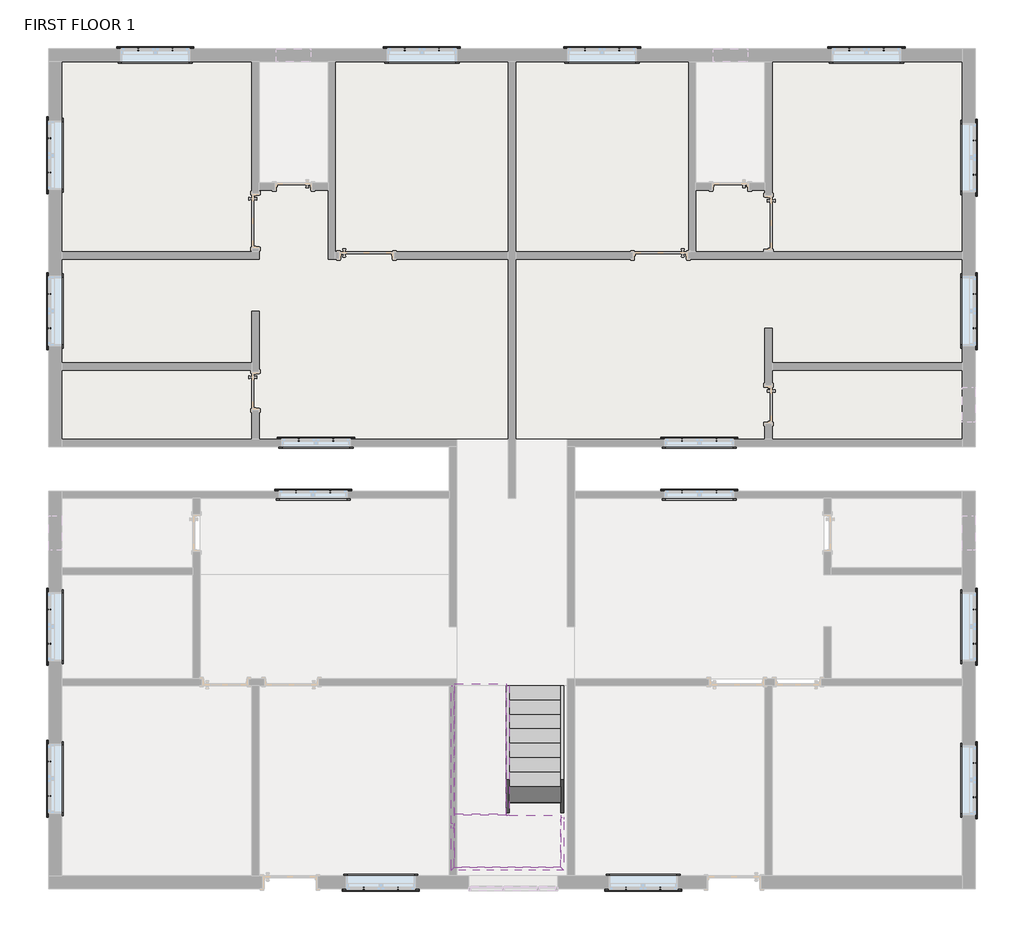
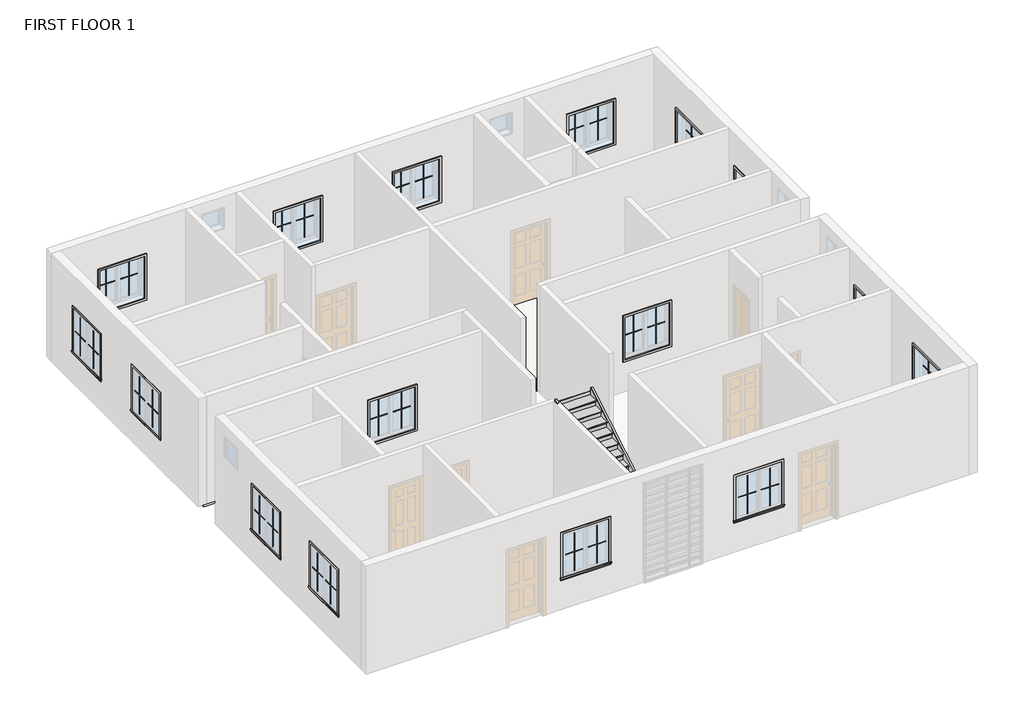
# One storey, part 4 of 4: 72 proxies, 7 members, 4 slabs, 2 stair flights.
"""IFC4 building model written with IfcOpenShell, lengths in millimetres."""

from ifc_helpers import new_model, si_unit, frame, origin, place, context, project, spatial, polyline, outline, extrude, faceted_brep, transform, mapped, element, save
from components import muntin_pattern_2x2_muntin_pattern_2x2_4dfeb3f3, muntin_pattern_2x2_muntin_pattern_2x2_e852a7e4, trim_window_exterior_flat_with_sill_7cfdd449, trim_window_interior_flat_picture_frame_f1e0b15b, non_monolithic_landing_7b61c384, stair_flight_f1905681, stair_flight_6110c9a1

model = new_model("IFC4")

# Units and contexts
model_context = context("Model", 3, world=origin())
ifc_project = project(units=[si_unit("LENGTHUNIT", "METRE", prefix="MILLI")], contexts=[model_context])

# Site, building, storey
site = spatial("IfcSite", under=ifc_project)
building = spatial("IfcBuilding", under=site)
storey = spatial("IfcBuildingStorey", under=building, Name="FIRST FLOOR 1", Elevation=3200.4)

# Proxies
placement = place(None, origin())
muntin_pattern_2x2_muntin_pattern_2x2_shape = muntin_pattern_2x2_muntin_pattern_2x2_4dfeb3f3(model_context)
element("IfcBuildingElementProxy", 1, Name="Muntin Pattern_2x2 : Muntin Pattern_2x2", ObjectType="Muntin Pattern_2x2 : Muntin Pattern_2x2", at=placement, inside=storey, context=model_context, shape_type="MappedRepresentation", body=[
    mapped(muntin_pattern_2x2_muntin_pattern_2x2_shape, transform((-12420.8887331, 2059.7281164, 4184.65), x_axis=(0.0, 1.0, 0.0), y_axis=(-1.0, 0.0, 0.0), z_axis=(0.0, 0.0, 1.0))),
])
element("IfcBuildingElementProxy", 2, Name="Muntin Pattern_2x2 : Muntin Pattern_2x2", ObjectType="Muntin Pattern_2x2 : Muntin Pattern_2x2", at=placement, inside=storey, context=model_context, shape_type="MappedRepresentation", body=[
    mapped(muntin_pattern_2x2_muntin_pattern_2x2_shape, transform((-12420.8887331, 4803.7218664, 4184.65), x_axis=(0.0, 1.0, 0.0), y_axis=(-1.0, 0.0, 0.0), z_axis=(0.0, 0.0, 1.0))),
])
element("IfcBuildingElementProxy", 3, Name="Muntin Pattern_2x2 : Muntin Pattern_2x2", ObjectType="Muntin Pattern_2x2 : Muntin Pattern_2x2", at=placement, inside=storey, context=model_context, shape_type="MappedRepresentation", body=[
    mapped(muntin_pattern_2x2_muntin_pattern_2x2_shape, transform((-10854.0262331, 6977.8031164, 4184.65), x_axis=(1.0, 0.0, 0.0), y_axis=(0.0, 1.0, 0.0), z_axis=(0.0, 0.0, 1.0))),
])
element("IfcBuildingElementProxy", 4, Name="Muntin Pattern_2x2 : Muntin Pattern_2x2", ObjectType="Muntin Pattern_2x2 : Muntin Pattern_2x2", at=placement, inside=storey, context=model_context, shape_type="MappedRepresentation", body=[
    mapped(muntin_pattern_2x2_muntin_pattern_2x2_shape, transform((-6155.0262331, 6977.8031164, 4184.65), x_axis=(1.0, 0.0, 0.0), y_axis=(0.0, 1.0, 0.0), z_axis=(0.0, 0.0, 1.0))),
])
element("IfcBuildingElementProxy", 5, Name="Muntin Pattern_2x2 : Muntin Pattern_2x2", ObjectType="Muntin Pattern_2x2 : Muntin Pattern_2x2", at=placement, inside=storey, context=model_context, shape_type="MappedRepresentation", body=[
    mapped(muntin_pattern_2x2_muntin_pattern_2x2_shape, transform((-2980.0262331, 6977.8031164, 4184.65), x_axis=(1.0, 0.0, 0.0), y_axis=(0.0, 1.0, 0.0), z_axis=(0.0, 0.0, 1.0))),
])
element("IfcBuildingElementProxy", 6, Name="Muntin Pattern_2x2 : Muntin Pattern_2x2", ObjectType="Muntin Pattern_2x2 : Muntin Pattern_2x2", at=placement, inside=storey, context=model_context, shape_type="MappedRepresentation", body=[
    mapped(muntin_pattern_2x2_muntin_pattern_2x2_shape, transform((1680.8737669, 6977.8031164, 4184.65), x_axis=(1.0, 0.0, 0.0), y_axis=(0.0, 1.0, 0.0), z_axis=(0.0, 0.0, 1.0))),
])
element("IfcBuildingElementProxy", 7, Name="Muntin Pattern_2x2 : Muntin Pattern_2x2", ObjectType="Muntin Pattern_2x2 : Muntin Pattern_2x2", at=placement, inside=storey, context=model_context, shape_type="MappedRepresentation", body=[
    mapped(muntin_pattern_2x2_muntin_pattern_2x2_shape, transform((3892.2612669, 5371.2531164, 4184.65), x_axis=(0.0, -1.0, 0.0), y_axis=(1.0, 0.0, 0.0), z_axis=(0.0, 0.0, 1.0))),
])
element("IfcBuildingElementProxy", 8, Name="Muntin Pattern_2x2 : Muntin Pattern_2x2", ObjectType="Muntin Pattern_2x2 : Muntin Pattern_2x2", at=placement, inside=storey, context=model_context, shape_type="MappedRepresentation", body=[
    mapped(muntin_pattern_2x2_muntin_pattern_2x2_shape, transform((3892.2612669, 2666.1531164, 4184.65), x_axis=(0.0, -1.0, 0.0), y_axis=(1.0, 0.0, 0.0), z_axis=(0.0, 0.0, 1.0))),
])
element("IfcBuildingElementProxy", 9, Name="Muntin Pattern_2x2 : Muntin Pattern_2x2", ObjectType="Muntin Pattern_2x2 : Muntin Pattern_2x2", at=placement, inside=storey, context=model_context, shape_type="MappedRepresentation", body=[
    mapped(muntin_pattern_2x2_muntin_pattern_2x2_shape, transform((3892.2612669, -2896.4468836, 4184.65), x_axis=(0.0, -1.0, 0.0), y_axis=(1.0, 0.0, 0.0), z_axis=(0.0, 0.0, 1.0))),
])
element("IfcBuildingElementProxy", 10, Name="Muntin Pattern_2x2 : Muntin Pattern_2x2", ObjectType="Muntin Pattern_2x2 : Muntin Pattern_2x2", at=placement, inside=storey, context=model_context, shape_type="MappedRepresentation", body=[
    mapped(muntin_pattern_2x2_muntin_pattern_2x2_shape, transform((3892.2612669, -5601.5468836, 4184.65), x_axis=(0.0, -1.0, 0.0), y_axis=(1.0, 0.0, 0.0), z_axis=(0.0, 0.0, 1.0))),
])
element("IfcBuildingElementProxy", 11, Name="Muntin Pattern_2x2 : Muntin Pattern_2x2", ObjectType="Muntin Pattern_2x2 : Muntin Pattern_2x2", at=placement, inside=storey, context=model_context, shape_type="MappedRepresentation", body=[
    mapped(muntin_pattern_2x2_muntin_pattern_2x2_shape, transform((-1649.7012331, -7812.9343836, 4184.65), x_axis=(-1.0, 0.0, 0.0), y_axis=(0.0, -1.0, 0.0), z_axis=(0.0, 0.0, 1.0))),
])
element("IfcBuildingElementProxy", 12, Name="Muntin Pattern_2x2 : Muntin Pattern_2x2", ObjectType="Muntin Pattern_2x2 : Muntin Pattern_2x2", at=placement, inside=storey, context=model_context, shape_type="MappedRepresentation", body=[
    mapped(muntin_pattern_2x2_muntin_pattern_2x2_shape, transform((-6272.5012331, -7812.9343836, 4184.65), x_axis=(-1.0, 0.0, 0.0), y_axis=(0.0, -1.0, 0.0), z_axis=(0.0, 0.0, 1.0))),
])
element("IfcBuildingElementProxy", 13, Name="Muntin Pattern_2x2 : Muntin Pattern_2x2", ObjectType="Muntin Pattern_2x2 : Muntin Pattern_2x2", at=placement, inside=storey, context=model_context, shape_type="MappedRepresentation", body=[
    mapped(muntin_pattern_2x2_muntin_pattern_2x2_shape, transform((-12420.8887331, -6182.5718836, 4184.65), x_axis=(0.0, 1.0, 0.0), y_axis=(-1.0, 0.0, 0.0), z_axis=(0.0, 0.0, 1.0))),
])
element("IfcBuildingElementProxy", 14, Name="Muntin Pattern_2x2 : Muntin Pattern_2x2", ObjectType="Muntin Pattern_2x2 : Muntin Pattern_2x2", at=placement, inside=storey, context=model_context, shape_type="MappedRepresentation", body=[
    mapped(muntin_pattern_2x2_muntin_pattern_2x2_shape, transform((-12420.8887331, -3502.8718836, 4184.65), x_axis=(0.0, 1.0, 0.0), y_axis=(-1.0, 0.0, 0.0), z_axis=(0.0, 0.0, 1.0))),
])
element("IfcBuildingElementProxy", 15, Name="Muntin Pattern_2x2 : Muntin Pattern_2x2", ObjectType="Muntin Pattern_2x2 : Muntin Pattern_2x2", at=placement, inside=storey, context=model_context, shape_type="MappedRepresentation", body=[
    mapped(muntin_pattern_2x2_muntin_pattern_2x2_shape, transform((-8072.7262331, -821.5843836, 4184.65), x_axis=(1.0, 0.0, 0.0), y_axis=(0.0, 1.0, 0.0), z_axis=(0.0, 0.0, 1.0))),
])
element("IfcBuildingElementProxy", 16, Name="Muntin Pattern_2x2 : Muntin Pattern_2x2", ObjectType="Muntin Pattern_2x2 : Muntin Pattern_2x2", at=placement, inside=storey, context=model_context, shape_type="MappedRepresentation", body=[
    mapped(muntin_pattern_2x2_muntin_pattern_2x2_shape, transform((-8021.9262331, 92.8156164, 4184.65), x_axis=(1.0, 0.0, 0.0), y_axis=(0.0, 1.0, 0.0), z_axis=(0.0, 0.0, 1.0))),
])
element("IfcBuildingElementProxy", 17, Name="Muntin Pattern_2x2 : Muntin Pattern_2x2", ObjectType="Muntin Pattern_2x2 : Muntin Pattern_2x2", at=placement, inside=storey, context=model_context, shape_type="MappedRepresentation", body=[
    mapped(muntin_pattern_2x2_muntin_pattern_2x2_shape, transform((-1265.5262331, -821.5843836, 4184.65), x_axis=(1.0, 0.0, 0.0), y_axis=(0.0, 1.0, 0.0), z_axis=(0.0, 0.0, 1.0))),
])
element("IfcBuildingElementProxy", 18, Name="Muntin Pattern_2x2 : Muntin Pattern_2x2", ObjectType="Muntin Pattern_2x2 : Muntin Pattern_2x2", at=placement, inside=storey, context=model_context, shape_type="MappedRepresentation", body=[
    mapped(muntin_pattern_2x2_muntin_pattern_2x2_shape, transform((-1265.5262331, 92.8156164, 4184.65), x_axis=(1.0, 0.0, 0.0), y_axis=(0.0, 1.0, 0.0), z_axis=(0.0, 0.0, 1.0))),
])
muntin_pattern_2x2_muntin_pattern_2x2_2_shape = muntin_pattern_2x2_muntin_pattern_2x2_e852a7e4(model_context)
element("IfcBuildingElementProxy", 19, Name="Muntin Pattern_2x2 : Muntin Pattern_2x2", ObjectType="Muntin Pattern_2x2 : Muntin Pattern_2x2", at=placement, inside=storey, context=model_context, shape_type="MappedRepresentation", body=[
    mapped(muntin_pattern_2x2_muntin_pattern_2x2_2_shape, transform((-12420.8887331, 2666.1531164, 4184.65), x_axis=(0.0, -1.0, 0.0), y_axis=(1.0, 0.0, 0.0), z_axis=(0.0, 0.0, 1.0))),
])
element("IfcBuildingElementProxy", 20, Name="Muntin Pattern_2x2 : Muntin Pattern_2x2", ObjectType="Muntin Pattern_2x2 : Muntin Pattern_2x2", at=placement, inside=storey, context=model_context, shape_type="MappedRepresentation", body=[
    mapped(muntin_pattern_2x2_muntin_pattern_2x2_2_shape, transform((-12420.8887331, 5410.1468664, 4184.65), x_axis=(0.0, -1.0, 0.0), y_axis=(1.0, 0.0, 0.0), z_axis=(0.0, 0.0, 1.0))),
])
element("IfcBuildingElementProxy", 21, Name="Muntin Pattern_2x2 : Muntin Pattern_2x2", ObjectType="Muntin Pattern_2x2 : Muntin Pattern_2x2", at=placement, inside=storey, context=model_context, shape_type="MappedRepresentation", body=[
    mapped(muntin_pattern_2x2_muntin_pattern_2x2_2_shape, transform((-10247.6012331, 6977.8031164, 4184.65), x_axis=(-1.0, 0.0, 0.0), y_axis=(0.0, -1.0, 0.0), z_axis=(0.0, 0.0, 1.0))),
])
element("IfcBuildingElementProxy", 22, Name="Muntin Pattern_2x2 : Muntin Pattern_2x2", ObjectType="Muntin Pattern_2x2 : Muntin Pattern_2x2", at=placement, inside=storey, context=model_context, shape_type="MappedRepresentation", body=[
    mapped(muntin_pattern_2x2_muntin_pattern_2x2_2_shape, transform((-5548.6012331, 6977.8031164, 4184.65), x_axis=(-1.0, 0.0, 0.0), y_axis=(0.0, -1.0, 0.0), z_axis=(0.0, 0.0, 1.0))),
])
element("IfcBuildingElementProxy", 23, Name="Muntin Pattern_2x2 : Muntin Pattern_2x2", ObjectType="Muntin Pattern_2x2 : Muntin Pattern_2x2", at=placement, inside=storey, context=model_context, shape_type="MappedRepresentation", body=[
    mapped(muntin_pattern_2x2_muntin_pattern_2x2_2_shape, transform((-2373.6012331, 6977.8031164, 4184.65), x_axis=(-1.0, 0.0, 0.0), y_axis=(0.0, -1.0, 0.0), z_axis=(0.0, 0.0, 1.0))),
])
element("IfcBuildingElementProxy", 24, Name="Muntin Pattern_2x2 : Muntin Pattern_2x2", ObjectType="Muntin Pattern_2x2 : Muntin Pattern_2x2", at=placement, inside=storey, context=model_context, shape_type="MappedRepresentation", body=[
    mapped(muntin_pattern_2x2_muntin_pattern_2x2_2_shape, transform((2287.2987669, 6977.8031164, 4184.65), x_axis=(-1.0, 0.0, 0.0), y_axis=(0.0, -1.0, 0.0), z_axis=(0.0, 0.0, 1.0))),
])
element("IfcBuildingElementProxy", 25, Name="Muntin Pattern_2x2 : Muntin Pattern_2x2", ObjectType="Muntin Pattern_2x2 : Muntin Pattern_2x2", at=placement, inside=storey, context=model_context, shape_type="MappedRepresentation", body=[
    mapped(muntin_pattern_2x2_muntin_pattern_2x2_2_shape, transform((3892.2612669, 4764.8281164, 4184.65), x_axis=(0.0, 1.0, 0.0), y_axis=(-1.0, 0.0, 0.0), z_axis=(0.0, 0.0, 1.0))),
])
element("IfcBuildingElementProxy", 26, Name="Muntin Pattern_2x2 : Muntin Pattern_2x2", ObjectType="Muntin Pattern_2x2 : Muntin Pattern_2x2", at=placement, inside=storey, context=model_context, shape_type="MappedRepresentation", body=[
    mapped(muntin_pattern_2x2_muntin_pattern_2x2_2_shape, transform((3892.2612669, 2059.7281164, 4184.65), x_axis=(0.0, 1.0, 0.0), y_axis=(-1.0, 0.0, 0.0), z_axis=(0.0, 0.0, 1.0))),
])
element("IfcBuildingElementProxy", 27, Name="Muntin Pattern_2x2 : Muntin Pattern_2x2", ObjectType="Muntin Pattern_2x2 : Muntin Pattern_2x2", at=placement, inside=storey, context=model_context, shape_type="MappedRepresentation", body=[
    mapped(muntin_pattern_2x2_muntin_pattern_2x2_2_shape, transform((3892.2612669, -3502.8718836, 4184.65), x_axis=(0.0, 1.0, 0.0), y_axis=(-1.0, 0.0, 0.0), z_axis=(0.0, 0.0, 1.0))),
])
element("IfcBuildingElementProxy", 28, Name="Muntin Pattern_2x2 : Muntin Pattern_2x2", ObjectType="Muntin Pattern_2x2 : Muntin Pattern_2x2", at=placement, inside=storey, context=model_context, shape_type="MappedRepresentation", body=[
    mapped(muntin_pattern_2x2_muntin_pattern_2x2_2_shape, transform((3892.2612669, -6207.9718836, 4184.65), x_axis=(0.0, 1.0, 0.0), y_axis=(-1.0, 0.0, 0.0), z_axis=(0.0, 0.0, 1.0))),
])
element("IfcBuildingElementProxy", 29, Name="Muntin Pattern_2x2 : Muntin Pattern_2x2", ObjectType="Muntin Pattern_2x2 : Muntin Pattern_2x2", at=placement, inside=storey, context=model_context, shape_type="MappedRepresentation", body=[
    mapped(muntin_pattern_2x2_muntin_pattern_2x2_2_shape, transform((-2256.1262331, -7812.9343836, 4184.65), x_axis=(1.0, 0.0, 0.0), y_axis=(0.0, 1.0, 0.0), z_axis=(0.0, 0.0, 1.0))),
])
element("IfcBuildingElementProxy", 30, Name="Muntin Pattern_2x2 : Muntin Pattern_2x2", ObjectType="Muntin Pattern_2x2 : Muntin Pattern_2x2", at=placement, inside=storey, context=model_context, shape_type="MappedRepresentation", body=[
    mapped(muntin_pattern_2x2_muntin_pattern_2x2_2_shape, transform((-6878.9262331, -7812.9343836, 4184.65), x_axis=(1.0, 0.0, 0.0), y_axis=(0.0, 1.0, 0.0), z_axis=(0.0, 0.0, 1.0))),
])
element("IfcBuildingElementProxy", 31, Name="Muntin Pattern_2x2 : Muntin Pattern_2x2", ObjectType="Muntin Pattern_2x2 : Muntin Pattern_2x2", at=placement, inside=storey, context=model_context, shape_type="MappedRepresentation", body=[
    mapped(muntin_pattern_2x2_muntin_pattern_2x2_2_shape, transform((-12420.8887331, -5576.1468836, 4184.65), x_axis=(0.0, -1.0, 0.0), y_axis=(1.0, 0.0, 0.0), z_axis=(0.0, 0.0, 1.0))),
])
element("IfcBuildingElementProxy", 32, Name="Muntin Pattern_2x2 : Muntin Pattern_2x2", ObjectType="Muntin Pattern_2x2 : Muntin Pattern_2x2", at=placement, inside=storey, context=model_context, shape_type="MappedRepresentation", body=[
    mapped(muntin_pattern_2x2_muntin_pattern_2x2_2_shape, transform((-12420.8887331, -2896.4468836, 4184.65), x_axis=(0.0, -1.0, 0.0), y_axis=(1.0, 0.0, 0.0), z_axis=(0.0, 0.0, 1.0))),
])
element("IfcBuildingElementProxy", 33, Name="Muntin Pattern_2x2 : Muntin Pattern_2x2", ObjectType="Muntin Pattern_2x2 : Muntin Pattern_2x2", at=placement, inside=storey, context=model_context, shape_type="MappedRepresentation", body=[
    mapped(muntin_pattern_2x2_muntin_pattern_2x2_2_shape, transform((-7466.3012331, -821.5843836, 4184.65), x_axis=(-1.0, 0.0, 0.0), y_axis=(0.0, -1.0, 0.0), z_axis=(0.0, 0.0, 1.0))),
])
element("IfcBuildingElementProxy", 34, Name="Muntin Pattern_2x2 : Muntin Pattern_2x2", ObjectType="Muntin Pattern_2x2 : Muntin Pattern_2x2", at=placement, inside=storey, context=model_context, shape_type="MappedRepresentation", body=[
    mapped(muntin_pattern_2x2_muntin_pattern_2x2_2_shape, transform((-7415.5012331, 92.8156164, 4184.65), x_axis=(-1.0, 0.0, 0.0), y_axis=(0.0, -1.0, 0.0), z_axis=(0.0, 0.0, 1.0))),
])
element("IfcBuildingElementProxy", 35, Name="Muntin Pattern_2x2 : Muntin Pattern_2x2", ObjectType="Muntin Pattern_2x2 : Muntin Pattern_2x2", at=placement, inside=storey, context=model_context, shape_type="MappedRepresentation", body=[
    mapped(muntin_pattern_2x2_muntin_pattern_2x2_2_shape, transform((-659.1012331, -821.5843836, 4184.65), x_axis=(-1.0, 0.0, 0.0), y_axis=(0.0, -1.0, 0.0), z_axis=(0.0, 0.0, 1.0))),
])
element("IfcBuildingElementProxy", 36, Name="Muntin Pattern_2x2 : Muntin Pattern_2x2", ObjectType="Muntin Pattern_2x2 : Muntin Pattern_2x2", at=placement, inside=storey, context=model_context, shape_type="MappedRepresentation", body=[
    mapped(muntin_pattern_2x2_muntin_pattern_2x2_2_shape, transform((-659.1012331, 92.8156164, 4184.65), x_axis=(-1.0, 0.0, 0.0), y_axis=(0.0, -1.0, 0.0), z_axis=(0.0, 0.0, 1.0))),
])
trim_window_exterior_flat_with_sill_shape = trim_window_exterior_flat_with_sill_7cfdd449(model_context)
element("IfcBuildingElementProxy", 37, Name="Trim-Window-Exterior-Flat : with Sill", ObjectType="Trim-Window-Exterior-Flat : with Sill", at=placement, inside=storey, context=model_context, shape_type="MappedRepresentation", body=[
    mapped(trim_window_exterior_flat_with_sill_shape, transform((-12430.4137331, 2362.9406164, 5334.0), x_axis=(0.0, -1.0, 0.0), y_axis=(0.0, 0.0, 1.0), z_axis=(-1.0, 0.0, 0.0))),
])
element("IfcBuildingElementProxy", 38, Name="Trim-Window-Exterior-Flat : with Sill", ObjectType="Trim-Window-Exterior-Flat : with Sill", at=placement, inside=storey, context=model_context, shape_type="MappedRepresentation", body=[
    mapped(trim_window_exterior_flat_with_sill_shape, transform((-12430.4137331, 5106.9343664, 5334.0), x_axis=(0.0, -1.0, 0.0), y_axis=(0.0, 0.0, 1.0), z_axis=(-1.0, 0.0, 0.0))),
])
element("IfcBuildingElementProxy", 39, Name="Trim-Window-Exterior-Flat : with Sill", ObjectType="Trim-Window-Exterior-Flat : with Sill", at=placement, inside=storey, context=model_context, shape_type="MappedRepresentation", body=[
    mapped(trim_window_exterior_flat_with_sill_shape, transform((-10550.8137331, 6987.3281164, 5334.0), x_axis=(-1.0, 0.0, 0.0), y_axis=(0.0, 0.0, 1.0), z_axis=(0.0, 1.0, 0.0))),
])
element("IfcBuildingElementProxy", 40, Name="Trim-Window-Exterior-Flat : with Sill", ObjectType="Trim-Window-Exterior-Flat : with Sill", at=placement, inside=storey, context=model_context, shape_type="MappedRepresentation", body=[
    mapped(trim_window_exterior_flat_with_sill_shape, transform((-5851.8137331, 6987.3281164, 5334.0), x_axis=(-1.0, 0.0, 0.0), y_axis=(0.0, 0.0, 1.0), z_axis=(0.0, 1.0, 0.0))),
])
element("IfcBuildingElementProxy", 41, Name="Trim-Window-Exterior-Flat : with Sill", ObjectType="Trim-Window-Exterior-Flat : with Sill", at=placement, inside=storey, context=model_context, shape_type="MappedRepresentation", body=[
    mapped(trim_window_exterior_flat_with_sill_shape, transform((-2676.8137331, 6987.3281164, 5334.0), x_axis=(-1.0, 0.0, 0.0), y_axis=(0.0, 0.0, 1.0), z_axis=(0.0, 1.0, 0.0))),
])
element("IfcBuildingElementProxy", 42, Name="Trim-Window-Exterior-Flat : with Sill", ObjectType="Trim-Window-Exterior-Flat : with Sill", at=placement, inside=storey, context=model_context, shape_type="MappedRepresentation", body=[
    mapped(trim_window_exterior_flat_with_sill_shape, transform((1984.0862669, 6987.3281164, 5334.0), x_axis=(-1.0, 0.0, 0.0), y_axis=(0.0, 0.0, 1.0), z_axis=(0.0, 1.0, 0.0))),
])
element("IfcBuildingElementProxy", 43, Name="Trim-Window-Exterior-Flat : with Sill", ObjectType="Trim-Window-Exterior-Flat : with Sill", at=placement, inside=storey, context=model_context, shape_type="MappedRepresentation", body=[
    mapped(trim_window_exterior_flat_with_sill_shape, transform((3901.7862669, 5068.0406164, 5334.0), x_axis=(0.0, 1.0, 0.0), y_axis=(0.0, 0.0, 1.0), z_axis=(1.0, 0.0, 0.0))),
])
element("IfcBuildingElementProxy", 44, Name="Trim-Window-Exterior-Flat : with Sill", ObjectType="Trim-Window-Exterior-Flat : with Sill", at=placement, inside=storey, context=model_context, shape_type="MappedRepresentation", body=[
    mapped(trim_window_exterior_flat_with_sill_shape, transform((3901.7862669, 2362.9406164, 5334.0), x_axis=(0.0, 1.0, 0.0), y_axis=(0.0, 0.0, 1.0), z_axis=(1.0, 0.0, 0.0))),
])
element("IfcBuildingElementProxy", 45, Name="Trim-Window-Exterior-Flat : with Sill", ObjectType="Trim-Window-Exterior-Flat : with Sill", at=placement, inside=storey, context=model_context, shape_type="MappedRepresentation", body=[
    mapped(trim_window_exterior_flat_with_sill_shape, transform((3901.7862669, -3199.6593836, 5334.0), x_axis=(0.0, 1.0, 0.0), y_axis=(0.0, 0.0, 1.0), z_axis=(1.0, 0.0, 0.0))),
])
element("IfcBuildingElementProxy", 46, Name="Trim-Window-Exterior-Flat : with Sill", ObjectType="Trim-Window-Exterior-Flat : with Sill", at=placement, inside=storey, context=model_context, shape_type="MappedRepresentation", body=[
    mapped(trim_window_exterior_flat_with_sill_shape, transform((3901.7862669, -5904.7593836, 5334.0), x_axis=(0.0, 1.0, 0.0), y_axis=(0.0, 0.0, 1.0), z_axis=(1.0, 0.0, 0.0))),
])
element("IfcBuildingElementProxy", 47, Name="Trim-Window-Exterior-Flat : with Sill", ObjectType="Trim-Window-Exterior-Flat : with Sill", at=placement, inside=storey, context=model_context, shape_type="MappedRepresentation", body=[
    mapped(trim_window_exterior_flat_with_sill_shape, transform((-1952.9137331, -7822.4593836, 5334.0), x_axis=(1.0, 0.0, 0.0), y_axis=(0.0, 0.0, 1.0), z_axis=(0.0, -1.0, 0.0))),
])
element("IfcBuildingElementProxy", 48, Name="Trim-Window-Exterior-Flat : with Sill", ObjectType="Trim-Window-Exterior-Flat : with Sill", at=placement, inside=storey, context=model_context, shape_type="MappedRepresentation", body=[
    mapped(trim_window_exterior_flat_with_sill_shape, transform((-6575.7137331, -7822.4593836, 5334.0), x_axis=(1.0, 0.0, 0.0), y_axis=(0.0, 0.0, 1.0), z_axis=(0.0, -1.0, 0.0))),
])
element("IfcBuildingElementProxy", 49, Name="Trim-Window-Exterior-Flat : with Sill", ObjectType="Trim-Window-Exterior-Flat : with Sill", at=placement, inside=storey, context=model_context, shape_type="MappedRepresentation", body=[
    mapped(trim_window_exterior_flat_with_sill_shape, transform((-12430.4137331, -5879.3593836, 5334.0), x_axis=(0.0, -1.0, 0.0), y_axis=(0.0, 0.0, 1.0), z_axis=(-1.0, 0.0, 0.0))),
])
element("IfcBuildingElementProxy", 50, Name="Trim-Window-Exterior-Flat : with Sill", ObjectType="Trim-Window-Exterior-Flat : with Sill", at=placement, inside=storey, context=model_context, shape_type="MappedRepresentation", body=[
    mapped(trim_window_exterior_flat_with_sill_shape, transform((-12430.4137331, -3199.6593836, 5334.0), x_axis=(0.0, -1.0, 0.0), y_axis=(0.0, 0.0, 1.0), z_axis=(-1.0, 0.0, 0.0))),
])
element("IfcBuildingElementProxy", 51, Name="Trim-Window-Exterior-Flat : with Sill", ObjectType="Trim-Window-Exterior-Flat : with Sill", at=placement, inside=storey, context=model_context, shape_type="MappedRepresentation", body=[
    mapped(trim_window_exterior_flat_with_sill_shape, transform((-7769.5137331, -812.0593836, 5334.0), x_axis=(-1.0, 0.0, 0.0), y_axis=(0.0, 0.0, 1.0), z_axis=(0.0, 1.0, 0.0))),
])
element("IfcBuildingElementProxy", 52, Name="Trim-Window-Exterior-Flat : with Sill", ObjectType="Trim-Window-Exterior-Flat : with Sill", at=placement, inside=storey, context=model_context, shape_type="MappedRepresentation", body=[
    mapped(trim_window_exterior_flat_with_sill_shape, transform((-7718.7137331, 102.3406164, 5334.0), x_axis=(-1.0, 0.0, 0.0), y_axis=(0.0, 0.0, 1.0), z_axis=(0.0, 1.0, 0.0))),
])
element("IfcBuildingElementProxy", 53, Name="Trim-Window-Exterior-Flat : with Sill", ObjectType="Trim-Window-Exterior-Flat : with Sill", at=placement, inside=storey, context=model_context, shape_type="MappedRepresentation", body=[
    mapped(trim_window_exterior_flat_with_sill_shape, transform((-962.3137331, -812.0593836, 5334.0), x_axis=(-1.0, 0.0, 0.0), y_axis=(0.0, 0.0, 1.0), z_axis=(0.0, 1.0, 0.0))),
])
element("IfcBuildingElementProxy", 54, Name="Trim-Window-Exterior-Flat : with Sill", ObjectType="Trim-Window-Exterior-Flat : with Sill", at=placement, inside=storey, context=model_context, shape_type="MappedRepresentation", body=[
    mapped(trim_window_exterior_flat_with_sill_shape, transform((-962.3137331, 102.3406164, 5334.0), x_axis=(-1.0, 0.0, 0.0), y_axis=(0.0, 0.0, 1.0), z_axis=(0.0, 1.0, 0.0))),
])
trim_window_interior_flat_picture_frame_shape = trim_window_interior_flat_picture_frame_f1e0b15b(model_context)
element("IfcBuildingElementProxy", 55, Name="Trim-Window-Interior-Flat : Picture Frame", ObjectType="Trim-Window-Interior-Flat : Picture Frame", at=placement, inside=storey, context=model_context, shape_type="MappedRepresentation", body=[
    mapped(trim_window_interior_flat_picture_frame_shape, transform((-12201.8137331, 2362.9406164, 5334.0), x_axis=(0.0, 1.0, 0.0), y_axis=(0.0, 0.0, 1.0), z_axis=(1.0, 0.0, 0.0))),
])
element("IfcBuildingElementProxy", 56, Name="Trim-Window-Interior-Flat : Picture Frame", ObjectType="Trim-Window-Interior-Flat : Picture Frame", at=placement, inside=storey, context=model_context, shape_type="MappedRepresentation", body=[
    mapped(trim_window_interior_flat_picture_frame_shape, transform((-12201.8137331, 5106.9343664, 5334.0), x_axis=(0.0, 1.0, 0.0), y_axis=(0.0, 0.0, 1.0), z_axis=(1.0, 0.0, 0.0))),
])
element("IfcBuildingElementProxy", 57, Name="Trim-Window-Interior-Flat : Picture Frame", ObjectType="Trim-Window-Interior-Flat : Picture Frame", at=placement, inside=storey, context=model_context, shape_type="MappedRepresentation", body=[
    mapped(trim_window_interior_flat_picture_frame_shape, transform((-10550.8137331, 6758.7281164, 5334.0), x_axis=(1.0, 0.0, 0.0), y_axis=(0.0, 0.0, 1.0), z_axis=(0.0, -1.0, 0.0))),
])
element("IfcBuildingElementProxy", 58, Name="Trim-Window-Interior-Flat : Picture Frame", ObjectType="Trim-Window-Interior-Flat : Picture Frame", at=placement, inside=storey, context=model_context, shape_type="MappedRepresentation", body=[
    mapped(trim_window_interior_flat_picture_frame_shape, transform((-5851.8137331, 6758.7281164, 5334.0), x_axis=(1.0, 0.0, 0.0), y_axis=(0.0, 0.0, 1.0), z_axis=(0.0, -1.0, 0.0))),
])
element("IfcBuildingElementProxy", 59, Name="Trim-Window-Interior-Flat : Picture Frame", ObjectType="Trim-Window-Interior-Flat : Picture Frame", at=placement, inside=storey, context=model_context, shape_type="MappedRepresentation", body=[
    mapped(trim_window_interior_flat_picture_frame_shape, transform((-2676.8137331, 6758.7281164, 5334.0), x_axis=(1.0, 0.0, 0.0), y_axis=(0.0, 0.0, 1.0), z_axis=(0.0, -1.0, 0.0))),
])
element("IfcBuildingElementProxy", 60, Name="Trim-Window-Interior-Flat : Picture Frame", ObjectType="Trim-Window-Interior-Flat : Picture Frame", at=placement, inside=storey, context=model_context, shape_type="MappedRepresentation", body=[
    mapped(trim_window_interior_flat_picture_frame_shape, transform((1984.0862669, 6758.7281164, 5334.0), x_axis=(1.0, 0.0, 0.0), y_axis=(0.0, 0.0, 1.0), z_axis=(0.0, -1.0, 0.0))),
])
element("IfcBuildingElementProxy", 61, Name="Trim-Window-Interior-Flat : Picture Frame", ObjectType="Trim-Window-Interior-Flat : Picture Frame", at=placement, inside=storey, context=model_context, shape_type="MappedRepresentation", body=[
    mapped(trim_window_interior_flat_picture_frame_shape, transform((3673.1862669, 5068.0406164, 5334.0), x_axis=(0.0, -1.0, 0.0), y_axis=(0.0, 0.0, 1.0), z_axis=(-1.0, 0.0, 0.0))),
])
element("IfcBuildingElementProxy", 62, Name="Trim-Window-Interior-Flat : Picture Frame", ObjectType="Trim-Window-Interior-Flat : Picture Frame", at=placement, inside=storey, context=model_context, shape_type="MappedRepresentation", body=[
    mapped(trim_window_interior_flat_picture_frame_shape, transform((3673.1862669, 2362.9406164, 5334.0), x_axis=(0.0, -1.0, 0.0), y_axis=(0.0, 0.0, 1.0), z_axis=(-1.0, 0.0, 0.0))),
])
element("IfcBuildingElementProxy", 63, Name="Trim-Window-Interior-Flat : Picture Frame", ObjectType="Trim-Window-Interior-Flat : Picture Frame", at=placement, inside=storey, context=model_context, shape_type="MappedRepresentation", body=[
    mapped(trim_window_interior_flat_picture_frame_shape, transform((3673.1862669, -3199.6593836, 5334.0), x_axis=(0.0, -1.0, 0.0), y_axis=(0.0, 0.0, 1.0), z_axis=(-1.0, 0.0, 0.0))),
])
element("IfcBuildingElementProxy", 64, Name="Trim-Window-Interior-Flat : Picture Frame", ObjectType="Trim-Window-Interior-Flat : Picture Frame", at=placement, inside=storey, context=model_context, shape_type="MappedRepresentation", body=[
    mapped(trim_window_interior_flat_picture_frame_shape, transform((3673.1862669, -5904.7593836, 5334.0), x_axis=(0.0, -1.0, 0.0), y_axis=(0.0, 0.0, 1.0), z_axis=(-1.0, 0.0, 0.0))),
])
element("IfcBuildingElementProxy", 65, Name="Trim-Window-Interior-Flat : Picture Frame", ObjectType="Trim-Window-Interior-Flat : Picture Frame", at=placement, inside=storey, context=model_context, shape_type="MappedRepresentation", body=[
    mapped(trim_window_interior_flat_picture_frame_shape, transform((-1952.9137331, -7593.8593836, 5334.0), x_axis=(-1.0, 0.0, 0.0), y_axis=(0.0, 0.0, 1.0), z_axis=(0.0, 1.0, 0.0))),
])
element("IfcBuildingElementProxy", 66, Name="Trim-Window-Interior-Flat : Picture Frame", ObjectType="Trim-Window-Interior-Flat : Picture Frame", at=placement, inside=storey, context=model_context, shape_type="MappedRepresentation", body=[
    mapped(trim_window_interior_flat_picture_frame_shape, transform((-6575.7137331, -7593.8593836, 5334.0), x_axis=(-1.0, 0.0, 0.0), y_axis=(0.0, 0.0, 1.0), z_axis=(0.0, 1.0, 0.0))),
])
element("IfcBuildingElementProxy", 67, Name="Trim-Window-Interior-Flat : Picture Frame", ObjectType="Trim-Window-Interior-Flat : Picture Frame", at=placement, inside=storey, context=model_context, shape_type="MappedRepresentation", body=[
    mapped(trim_window_interior_flat_picture_frame_shape, transform((-12201.8137331, -5879.3593836, 5334.0), x_axis=(0.0, 1.0, 0.0), y_axis=(0.0, 0.0, 1.0), z_axis=(1.0, 0.0, 0.0))),
])
element("IfcBuildingElementProxy", 68, Name="Trim-Window-Interior-Flat : Picture Frame", ObjectType="Trim-Window-Interior-Flat : Picture Frame", at=placement, inside=storey, context=model_context, shape_type="MappedRepresentation", body=[
    mapped(trim_window_interior_flat_picture_frame_shape, transform((-12201.8137331, -3199.6593836, 5334.0), x_axis=(0.0, 1.0, 0.0), y_axis=(0.0, 0.0, 1.0), z_axis=(1.0, 0.0, 0.0))),
])
element("IfcBuildingElementProxy", 69, Name="Trim-Window-Interior-Flat : Picture Frame", ObjectType="Trim-Window-Interior-Flat : Picture Frame", at=placement, inside=storey, context=model_context, shape_type="MappedRepresentation", body=[
    mapped(trim_window_interior_flat_picture_frame_shape, transform((-7769.5137331, -939.0593836, 5334.0), x_axis=(1.0, 0.0, 0.0), y_axis=(0.0, 0.0, 1.0), z_axis=(0.0, -1.0, 0.0))),
])
element("IfcBuildingElementProxy", 70, Name="Trim-Window-Interior-Flat : Picture Frame", ObjectType="Trim-Window-Interior-Flat : Picture Frame", at=placement, inside=storey, context=model_context, shape_type="MappedRepresentation", body=[
    mapped(trim_window_interior_flat_picture_frame_shape, transform((-7718.7137331, -24.6593836, 5334.0), x_axis=(1.0, 0.0, 0.0), y_axis=(0.0, 0.0, 1.0), z_axis=(0.0, -1.0, 0.0))),
])
element("IfcBuildingElementProxy", 71, Name="Trim-Window-Interior-Flat : Picture Frame", ObjectType="Trim-Window-Interior-Flat : Picture Frame", at=placement, inside=storey, context=model_context, shape_type="MappedRepresentation", body=[
    mapped(trim_window_interior_flat_picture_frame_shape, transform((-962.3137331, -939.0593836, 5334.0), x_axis=(1.0, 0.0, 0.0), y_axis=(0.0, 0.0, 1.0), z_axis=(0.0, -1.0, 0.0))),
])
element("IfcBuildingElementProxy", 72, Name="Trim-Window-Interior-Flat : Picture Frame", ObjectType="Trim-Window-Interior-Flat : Picture Frame", at=placement, inside=storey, context=model_context, shape_type="MappedRepresentation", body=[
    mapped(trim_window_interior_flat_picture_frame_shape, transform((-962.3137331, -24.6593836, 5334.0), x_axis=(1.0, 0.0, 0.0), y_axis=(0.0, 0.0, 1.0), z_axis=(0.0, -1.0, 0.0))),
])

# Members
element("IfcMember", 73, ObjectType="Stringer - 2\" Width", at=placement, inside=storey, context=model_context, shape_type="SweptSolid", body=[
    extrude(outline(polyline([(-4241.0593836, 3411.9517384), (-4241.0593836, 3200.4), (-4480.8978654, 3200.4), (-6639.8978654, 4495.8), (-6555.4731529, 4800.6), (-4241.0593836, 3411.9517384)])), frame((-3400.7137331, 0.0, 0.0), z_axis=(1.0, 0.0, 0.0), x_axis=(0.0, 1.0, 0.0)), (0.0, 0.0, 1.0), 50.8),
])
element("IfcMember", 74, ObjectType="Stringer - 2\" Width", at=placement, inside=storey, context=model_context, shape_type="SweptSolid", body=[
    extrude(outline(polyline([(-4241.0593836, 3411.9517384), (-4241.0593836, 3200.4), (-4480.8978654, 3200.4), (-6476.2593836, 4397.6169109), (-6476.2593836, 4753.0717384), (-4241.0593836, 3411.9517384)])), frame((-4365.9137331, 0.0, 0.0), z_axis=(1.0, 0.0, 0.0), x_axis=(0.0, 1.0, 0.0)), (0.0, 0.0, 1.0), 50.8),
])
element("IfcMember", 75, ObjectType="Stringer - 2\" Width", at=placement, inside=storey, context=model_context, shape_type="SweptSolid", body=[
    extrude(outline(polyline([(-6668.2209018, 4495.8), (-6752.6456143, 4800.6), (-4241.0593836, 6307.5517384), (-4241.0593836, 5952.0969109), (-6668.2209018, 4495.8)])), frame((-5331.1137331, 0.0, 0.0), z_axis=(1.0, 0.0, 0.0), x_axis=(0.0, 1.0, 0.0)), (0.0, 0.0, 1.0), 50.8),
])
element("IfcMember", 76, ObjectType="Stringer - 2\" Width", at=placement, inside=storey, context=model_context, shape_type="SweptSolid", body=[
    extrude(outline(polyline([(-6527.0593836, 4580.4969109), (-6527.0593836, 4935.9517384), (-4241.0593836, 6307.5517384), (-4241.0593836, 5952.0969109), (-6527.0593836, 4580.4969109)])), frame((-4365.9137331, 0.0, 0.0), z_axis=(1.0, 0.0, 0.0), x_axis=(0.0, 1.0, 0.0)), (0.0, 0.0, 1.0), 50.8),
])
element("IfcMember", 77, ObjectType="Stringer - 2\" Width", at=placement, inside=storey, context=model_context, shape_type="Brep", body=[
    faceted_brep([(-5280.3137331, -6752.6456143, 4800.6), (-5331.1137331, -6752.6456143, 4800.6), (-5331.1137331, -7492.2593836, 4800.6), (-5280.3137331, -7441.4593836, 4800.6), (-5280.3137331, -6668.2209018, 4495.8), (-5280.3137331, -7441.4593836, 4495.8), (-5331.1137331, -6668.2209018, 4495.8), (-5331.1137331, -7492.2593836, 4495.8)], [[[0, 1, 2, 3]], [[4, 0, 3, 5]], [[6, 4, 5, 7]], [[1, 6, 7, 2]], [[1, 0, 4, 6]], [[2, 7, 5, 3]]]),
])
element("IfcMember", 78, ObjectType="Stringer - 2\" Width", at=placement, inside=storey, context=model_context, shape_type="SweptSolid", body=[
    extrude(outline(polyline([(-5331.1137331, -7492.2593836), (-5280.3137331, -7441.4593836), (-3400.7137331, -7441.4593836), (-3349.9137331, -7492.2593836), (-5331.1137331, -7492.2593836)])), frame((0.0, 0.0, 4495.8), z_axis=(0.0, 0.0, 1.0), x_axis=(1.0, 0.0, 0.0)), (0.0, 0.0, 1.0), 304.8),
])
element("IfcMember", 79, ObjectType="Stringer - 2\" Width", at=placement, inside=storey, context=model_context, shape_type="Brep", body=[
    faceted_brep([(-3400.7137331, -7441.4593836, 4800.6), (-3349.9137331, -7492.2593836, 4800.6), (-3349.9137331, -6555.4731529, 4800.6), (-3400.7137331, -6555.4731529, 4800.6), (-3400.7137331, -7441.4593836, 4495.8), (-3400.7137331, -6639.8978654, 4495.8), (-3349.9137331, -7492.2593836, 4495.8), (-3349.9137331, -6639.8978654, 4495.8)], [[[0, 1, 2, 3]], [[4, 0, 3, 5]], [[6, 4, 5, 7]], [[1, 6, 7, 2]], [[1, 0, 4, 6]], [[2, 7, 5, 3]]]),
])

# Slabs
non_monolithic_landing_shape = non_monolithic_landing_7b61c384(model_context)
element("IfcSlab", 80, ObjectType="Non-Monolithic Landing", at=placement, inside=storey, context=model_context, shape_type="MappedRepresentation", body=[
    mapped(non_monolithic_landing_shape, transform((0.0, 0.0, 0.0), x_axis=(1.0, 0.0, 0.0), y_axis=(0.0, 1.0, 0.0), z_axis=(0.0, 0.0, 1.0))),
])
element("IfcSlab", 81, ObjectType="marble tiles", at=placement, inside=storey, context=model_context, shape_type="SweptSolid", body=[
    extrude(outline(polyline([(3673.1862669, 102.3406164), (-12201.8137331, 102.3406164), (-12201.8137331, 6758.7281164), (3673.1862669, 6758.7281164), (3673.1862669, 102.3406164)])), frame((0.0, 0.0, 3048.0), z_axis=(0.0, 0.0, 1.0), x_axis=(1.0, 0.0, 0.0)), (0.0, 0.0, 1.0), 152.4),
])
element("IfcSlab", 82, ObjectType="marble tiles", at=placement, inside=storey, context=model_context, shape_type="SweptSolid", body=[
    extrude(outline(polyline([(-9890.4137331, -939.0593836), (-9890.4137331, -2158.2593836), (-12201.8137331, -2158.2593836), (-12201.8137331, -939.0593836), (-9890.4137331, -939.0593836)])), frame((0.0, 0.0, 3048.0), z_axis=(0.0, 0.0, 1.0), x_axis=(1.0, 0.0, 0.0)), (0.0, 0.0, 1.0), 152.4),
    extrude(outline(polyline([(3673.1862669, -2158.2593836), (1361.7862669, -2158.2593836), (1361.7862669, -939.0593836), (3673.1862669, -939.0593836), (3673.1862669, -2158.2593836)])), frame((0.0, 0.0, 3048.0), z_axis=(0.0, 0.0, 1.0), x_axis=(1.0, 0.0, 0.0)), (0.0, 0.0, 1.0), 152.4),
    extrude(outline(polyline([(-7502.8137331, 6758.7281164), (-7502.8137331, 4623.5406164), (-8722.0137331, 4623.5406164), (-8722.0137331, 6758.7281164), (-7502.8137331, 6758.7281164)])), frame((0.0, 0.0, 3048.0), z_axis=(0.0, 0.0, 1.0), x_axis=(1.0, 0.0, 0.0)), (0.0, 0.0, 1.0), 152.4),
    extrude(outline(polyline([(193.3862669, 4623.5406164), (-1025.8137331, 4623.5406164), (-1025.8137331, 6758.7281164), (193.3862669, 6758.7281164), (193.3862669, 4623.5406164)])), frame((0.0, 0.0, 3048.0), z_axis=(0.0, 0.0, 1.0), x_axis=(1.0, 0.0, 0.0)), (0.0, 0.0, 1.0), 152.4),
])
element("IfcSlab", 83, ObjectType="marble tiles", at=placement, inside=storey, context=model_context, shape_type="SweptSolid", body=[
    extrude(outline(polyline([(3673.1862669, 102.3406164), (-12201.8137331, 102.3406164), (-12201.8137331, 6758.7281164), (3673.1862669, 6758.7281164), (3673.1862669, 102.3406164)])), frame((0.0, 0.0, 3048.0), z_axis=(0.0, 0.0, 1.0), x_axis=(1.0, 0.0, 0.0)), (0.0, 0.0, 1.0), 152.4),
])

# Stair flights
stair_flight_shape = stair_flight_f1905681(model_context)
element("IfcStairFlight", 84, ObjectType="2\" Tread 1\" Nosing 1/4\" Riser", at=placement, inside=storey, context=model_context, shape_type="MappedRepresentation", body=[
    mapped(stair_flight_shape, transform((0.0, 0.0, 0.0), x_axis=(1.0, 0.0, 0.0), y_axis=(0.0, 1.0, 0.0), z_axis=(0.0, 0.0, 1.0))),
])
stair_flight_2_shape = stair_flight_6110c9a1(model_context)
element("IfcStairFlight", 85, ObjectType="2\" Tread 1\" Nosing 1/4\" Riser", at=placement, inside=storey, context=model_context, shape_type="MappedRepresentation", body=[
    mapped(stair_flight_2_shape, transform((0.0, 0.0, 0.0), x_axis=(1.0, 0.0, 0.0), y_axis=(0.0, 1.0, 0.0), z_axis=(0.0, 0.0, 1.0))),
])

save(model, "model.ifc")

# Revit data of these elements
# Type "Muntin Pattern_2x2 : Muntin Pattern_2x2"
#   Width [instance default] = 4' - 0"
#   Thickness = 0' - 0 1/2"
#   Height [instance default] = 4' - 0"
#   Distance = 0' - 0 3/4"
#   Interior Material [instance default] = none
#   Exterior Material [instance default] = none
#   Default Elevation = 0
# Type "Trim-Window-Exterior-Flat : with Sill"
#   Trim Width = 0' - 2 1/4"
#   Trim Thickness_Picture Frame = 0' - 1 1/4"
#   Trim Thickness_with Sill = 0' - 0 3/4"
#   Sill Thickness = 0' - 1 1/4"
#   Opening Width [instance default] = 2' - 0"
#   Opening Height [instance default] = 3' - 0"
#   Default Elevation = 4' - 0"
#   Sill = yes
#   Picture Frame = no
#   Trim Material [instance default] = none
# Type "Trim-Window-Interior-Flat : Picture Frame"
#   Trim Thickness_Picture Frame = 0' - 1 1/4"
#   Trim Width = 0' - 2 1/4"
#   Trim Thickness_with Sill = 0' - 0 3/4"
#   Sill Thickness = 0' - 1 1/4"
#   Opening Width [instance default] = 2' - 0"
#   Opening Height [instance default] = 3' - 0"
#   Default Elevation = 4' - 0"
#   Sill = no
#   Picture Frame = yes
#   Trim Material [instance default] = none
# Type "marble tiles"
#   Assembly Code = "B1010"
#   Function = 0
#   Layers, outside or top first: 0' - 6" "marble flooring" (function 1)
# Elements 1, 2, 3, 4, 5, 6, 7, 8, 9, 10, 11, 12, 13, 14, 15, 16, 17, 18, 19, 20, 21, 22, 23, 24, 25, 26, 27, 28, 29, 30, 31, 32, 33, 34, 35, 36 (IfcBuildingElementProxy, "Muntin Pattern_2x2 : Muntin Pattern_2x2")
#   Width = 1' - 6 5/8"
#   Height = 3' - 6 1/2"
#   Interior Material = Wood - Stained
#   Exterior Material = Clad - White
#   Phase Created = New Construction
#   Materials on its faces: "Clad - White", "Wood - Stained"
# Elements 37, 38, 39, 40, 41, 42, 43, 44, 45, 46, 47, 48, 49, 50, 51, 52, 53, 54 (IfcBuildingElementProxy, "Trim-Window-Exterior-Flat : with Sill")
#   Opening Width = 4' - 0"
#   Opening Height = 4' - 0"
#   Trim Material = Clad - White
#   Phase Created = New Construction
#   Materials on its faces: "Clad - White"
# Elements 55, 56, 57, 58, 59, 60, 61, 62, 63, 64, 65, 66, 67, 68, 69, 70, 71, 72 (IfcBuildingElementProxy, "Trim-Window-Interior-Flat : Picture Frame")
#   Opening Width = 4' - 0"
#   Opening Height = 4' - 0"
#   Trim Material = Wood - Stained
#   Phase Created = New Construction
#   Materials on its faces: "Wood - Stained"
# Elements 73, 74, 75, 76, 77, 78, 79 (IfcMember, "Stringer - 2\" Width")
#   Phase Created = New Construction
# Element 80 (IfcSlab, "Non-Monolithic Landing")
#   Phase Created = New Construction
# Elements 81, 82, 83 (IfcSlab, "marble tiles")
#   Height Offset From Level = 0' - 0"
#   Phase Created = New Construction
#   Materials on its faces: "marble flooring"
# Elements 84, 85 (IfcStairFlight, "2\" Tread 1\" Nosing 1/4\" Riser")
#   Phase Created = New Construction
# Materials
#   "marble flooring": class "Generic", colour RGB 120 120 120, transparency 0, Cost = 0
#   "Clad - White": class "Wood", colour RGB 242 242 238, transparency 0, Cost = 0
#   "Wood - Stained": class "Wood", colour RGB 224 178 126, transparency 0, Cost = 0
